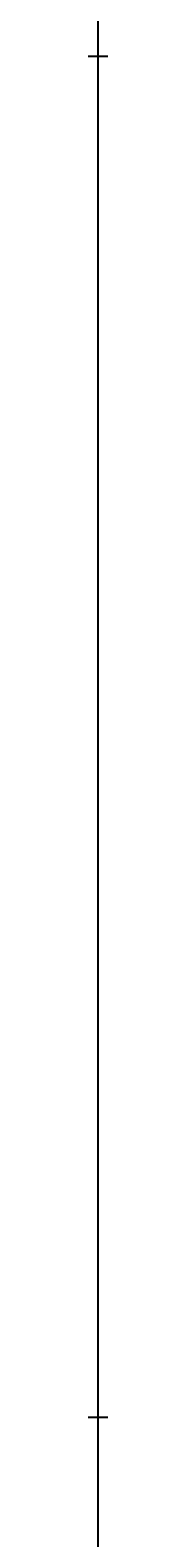
# Model space of a CAD drawing. Units: inches. Extents: x 35362 to 73946, y 43607 to 67532.
# Tile 42 of 134: x 48374 to 48374, y 46091 to 46564. Entities that reach past the tile are written whole.
import ezdxf

# ---------------------------------------------------------------- set-up
doc = ezdxf.new("R2010")
doc.units = ezdxf.units.IN
doc.header["$MEASUREMENT"] = 0
doc.layers.add('A-ANNO-DIMS', color=2, linetype='Continuous', lineweight=18)
doc.styles.get("Standard").update_dxf_attribs({"font": 'arial.ttf'})
doc.dimstyles.get("Standard").update_dxf_attribs({"dimtxt": 0.18, "dimasz": 0.18, "dimexe": 0.18, "dimexo": 0.0625, "dimgap": 0.09, "dimtad": 0, "dimtih": 1, "dimtoh": 1, "dimdec": 4, "dimzin": 0, "dimdsep": 46, "dimtxsty": 'Standard', "dimcen": 0.09, "dimadec": 0, "dimazin": 0, "dimtfac": 1, "dimtdec": 4, "dimtofl": 0, "dimtmove": 0, "dimatfit": 3, "dimfxl": 1, "dimtolj": 1, "dimtzin": 0, "dimarcsym": 0})

# ---------------------------------------------------------------- blocks, each defined once
blk = doc.blocks.new('*D5')
at = {"layer": 'A-ANNO-DIMS', "color": 0, "lineweight": -2, "transparency": 16777216}
for p, q in [((37121.95, 46919.32), (37121.95, 43606.68)), ((69871.5, 45449.83), (69871.5, 43606.68)), ((37122.13, 43606.86), (53496.29, 43606.86)), ((69871.32, 43606.86), (53497.15, 43606.86))]:
    blk.add_line(p, q, dxfattribs=at)
at = {"layer": 'A-ANNO-DIMS', "color": 0, "transparency": 16777216}
for points in [[(37122.13, 43606.89), (37122.13, 43606.83), (37121.95, 43606.86)], [(69871.32, 43606.89), (69871.32, 43606.83), (69871.5, 43606.86)]]:
    blk.add_solid(points, dxfattribs=at)
at = {"layer": 'Defpoints', "color": 0, "transparency": 16777216}
for p in [(37121.95, 46919.38), (69871.5, 45449.89), (69871.5, 43606.86)]:
    blk.add_point(p, dxfattribs=at)
at = {"layer": 'A-ANNO-DIMS', "color": 0, "transparency": 16777216, "insert": (53496.72, 43606.86), "char_height": 0.18, "attachment_point": 5}
blk.add_mtext('\\A1;32750', dxfattribs=at)
blk = doc.blocks.new('*D11')
at = {"layer": 'A-ANNO-DIMS', "color": 0, "lineweight": -2, "transparency": 16777216}
for p, q in [((47978.66, 56028.77), (47978.66, 43606.68)), ((53109.76, 56028.77), (53109.76, 43606.68)), ((47978.84, 43606.86), (50543.87, 43606.86)), ((53109.58, 43606.86), (50544.55, 43606.86))]:
    blk.add_line(p, q, dxfattribs=at)
at = {"layer": 'A-ANNO-DIMS', "color": 0, "transparency": 16777216}
for points in [[(47978.84, 43606.89), (47978.84, 43606.83), (47978.66, 43606.86)], [(53109.58, 43606.89), (53109.58, 43606.83), (53109.76, 43606.86)]]:
    blk.add_solid(points, dxfattribs=at)
at = {"layer": 'Defpoints', "color": 0, "transparency": 16777216}
for p in [(47978.66, 56028.84), (53109.76, 56028.84), (53109.76, 43606.86)]:
    blk.add_point(p, dxfattribs=at)
at = {"layer": 'A-ANNO-DIMS', "color": 0, "transparency": 16777216, "insert": (50544.21, 43606.86), "char_height": 0.18, "attachment_point": 5}
blk.add_mtext('\\A1;5131', dxfattribs=at)
blk = doc.blocks.new('*D13')
at = {"layer": 'A-ANNO-DIMS', "color": 0, "lineweight": -2, "transparency": 16777216}
for p, q in [((48373.49, 51694.02), (48373.49, 43606.68)), ((51029.04, 51694.02), (51029.04, 43606.68)), ((48373.67, 43606.86), (49700.8, 43606.86)), ((51028.86, 43606.86), (49701.73, 43606.86))]:
    blk.add_line(p, q, dxfattribs=at)
at = {"layer": 'A-ANNO-DIMS', "color": 0, "transparency": 16777216}
for points in [[(48373.67, 43606.89), (48373.67, 43606.83), (48373.49, 43606.86)], [(51028.86, 43606.89), (51028.86, 43606.83), (51029.04, 43606.86)]]:
    blk.add_solid(points, dxfattribs=at)
at = {"layer": 'Defpoints', "color": 0, "transparency": 16777216}
for p in [(48373.49, 51694.09), (51029.04, 51694.09), (51029.04, 43606.86)]:
    blk.add_point(p, dxfattribs=at)
at = {"layer": 'A-ANNO-DIMS', "color": 0, "transparency": 16777216, "insert": (49701.27, 43606.86), "char_height": 0.18, "attachment_point": 5}
blk.add_mtext('\\A1;2655.6', dxfattribs=at)
blk = doc.blocks.new('*D67')
at = {"layer": 'A-ANNO-DIMS', "color": 0, "lineweight": -2, "transparency": 16777216}
for p, q in [((56873.54, 53351.53), (35361.77, 53351.53)), ((35361.95, 53351.35), (35361.95, 49400.89)), ((35361.95, 45450.07), (35361.95, 49400.53)), ((53793.58, 45449.89), (35361.77, 45449.89))]:
    blk.add_line(p, q, dxfattribs=at)
at = {"layer": 'A-ANNO-DIMS', "color": 0, "transparency": 16777216}
for points in [[(35361.92, 53351.35), (35361.98, 53351.35), (35361.95, 53351.53)], [(35361.92, 45450.07), (35361.98, 45450.07), (35361.95, 45449.89)]]:
    blk.add_solid(points, dxfattribs=at)
at = {"layer": 'Defpoints', "color": 0, "transparency": 16777216}
for p in [(35361.95, 53351.53), (56873.6, 53351.53), (53793.64, 45449.89)]:
    blk.add_point(p, dxfattribs=at)
at = {"layer": 'A-ANNO-DIMS', "color": 0, "transparency": 16777216, "insert": (35361.95, 49400.71), "char_height": 0.18, "attachment_point": 5}
blk.add_mtext('\\A1;7901.6', dxfattribs=at)
blk = doc.blocks.new('*D76')
at = {"layer": 'A-ANNO-DIMS', "color": 0, "lineweight": -2, "transparency": 16777216}
for p, q in [((54052.84, 46555.29), (35361.77, 46555.29)), ((35361.95, 46555.11), (35361.95, 46342.27)), ((35361.95, 46129.06), (35361.95, 46341.9)), ((53793.58, 46128.88), (35361.77, 46128.88))]:
    blk.add_line(p, q, dxfattribs=at)
at = {"layer": 'A-ANNO-DIMS', "color": 0, "transparency": 16777216}
for points in [[(35361.92, 46555.11), (35361.98, 46555.11), (35361.95, 46555.29)], [(35361.92, 46129.06), (35361.98, 46129.06), (35361.95, 46128.88)]]:
    blk.add_solid(points, dxfattribs=at)
at = {"layer": 'Defpoints', "color": 0, "transparency": 16777216}
for p in [(35361.95, 46555.29), (54052.9, 46555.29), (53793.64, 46128.88)]:
    blk.add_point(p, dxfattribs=at)
at = {"layer": 'A-ANNO-DIMS', "color": 0, "transparency": 16777216, "insert": (35361.95, 46342.09), "char_height": 0.18, "attachment_point": 5}
blk.add_mtext('\\A1;426.4', dxfattribs=at)
blk = doc.blocks.new('*D90')
at = {"layer": 'A-ANNO-DIMS', "color": 0, "lineweight": -2, "transparency": 16777216}
for p, q in [((53707.72, 47291.29), (35361.77, 47291.29)), ((35361.95, 47291.11), (35361.95, 46710.26)), ((35361.95, 46129.06), (35361.95, 46709.9)), ((53793.58, 46128.88), (35361.77, 46128.88))]:
    blk.add_line(p, q, dxfattribs=at)
at = {"layer": 'A-ANNO-DIMS', "color": 0, "transparency": 16777216}
for points in [[(35361.92, 47291.11), (35361.98, 47291.11), (35361.95, 47291.29)], [(35361.92, 46129.06), (35361.98, 46129.06), (35361.95, 46128.88)]]:
    blk.add_solid(points, dxfattribs=at)
at = {"layer": 'Defpoints', "color": 0, "transparency": 16777216}
for p in [(53707.78, 47291.29), (35361.95, 46128.88), (53793.64, 46128.88)]:
    blk.add_point(p, dxfattribs=at)
at = {"layer": 'A-ANNO-DIMS', "color": 0, "transparency": 16777216, "insert": (35361.95, 46710.08), "char_height": 0.18, "attachment_point": 5}
blk.add_mtext('\\A1;1162.4', dxfattribs=at)

msp = doc.modelspace()

# ---------------------------------------------------------------- dimensions: what is measured, and where the dimension line sits
at = {"layer": 'A-ANNO-DIMS'}
for base, p1, p2, override, picture, middle in [((53109.76, 43606.859), (47978.665, 56028.836), (53109.76, 56028.836), {"dimdec": 0, "dimlfac": 1, "dimrnd": 0, "dimzin": 0, "dimdsep": 46, "dimlunit": 2}, '*D11', (50544.212, 43606.859)), ((51029.043, 43606.859), (48373.492, 51694.087), (51029.043, 51694.087), {"dimdec": 1, "dimlfac": 1, "dimrnd": 0, "dimzin": 0, "dimdsep": 46, "dimlunit": 2}, '*D13', (49701.267, 43606.859)), ((69871.496, 43606.859), (37121.949, 46919.381), (69871.496, 45449.894), {"dimdec": 0, "dimlfac": 1, "dimrnd": 0, "dimzin": 0, "dimdsep": 46, "dimlunit": 2}, '*D5', (53496.723, 43606.859))]:
    dim = msp.add_linear_dim(base=base, p1=p1, p2=p2, dimstyle='Standard', override=override, dxfattribs=at)
    dim.commit()
    dim.dimension.update_dxf_attribs({"geometry": picture, "text_midpoint": middle})
for base, p1, p2, picture, middle in [((35361.949, 53351.529), (53793.638, 45449.894), (56873.602, 53351.529), '*D67', (35361.949, 49400.712)), ((35361.949, 46128.878), (53707.781, 47291.285), (53793.638, 46128.878), '*D90', (35361.949, 46710.081)), ((35361.949, 46555.293), (53793.638, 46128.878), (54052.899, 46555.293), '*D76', (35361.949, 46342.086))]:
    dim = msp.add_linear_dim(base=base, p1=p1, p2=p2, angle=90, dimstyle='Standard', override={"dimdec": 1, "dimlfac": 1, "dimrnd": 0, "dimzin": 0, "dimdsep": 46, "dimlunit": 2}, dxfattribs=at)
    dim.commit()
    dim.dimension.update_dxf_attribs({"geometry": picture, "text_midpoint": middle})

doc.saveas('drawing.dxf')
